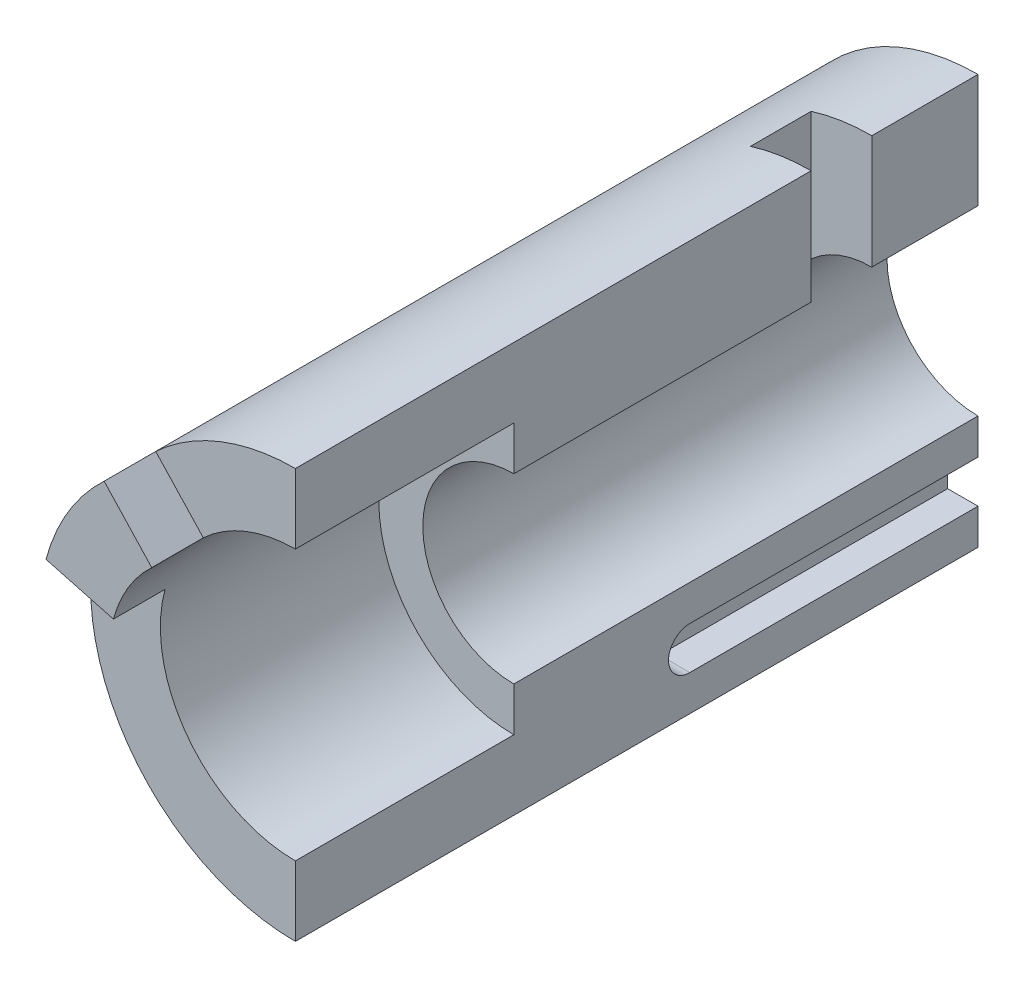
ISO-10303-21;
HEADER;
FILE_DESCRIPTION(('STEP AP214'),'2;1');
FILE_NAME('part.step','',(''),(''),'','','');
FILE_SCHEMA(('AUTOMOTIVE_DESIGN { 1 0 10303 214 1 1 1 1 }'));
ENDSEC;
DATA;
#1=APPLICATION_CONTEXT('core data for automotive mechanical design processes');
#2=APPLICATION_PROTOCOL_DEFINITION('international standard','automotive_design',2000,#1);
#3=PRODUCT_CONTEXT('',#1,'mechanical');
#4=PRODUCT('Part','Part','',(#3));
#5=PRODUCT_RELATED_PRODUCT_CATEGORY('part','',(#4));
#6=PRODUCT_DEFINITION_FORMATION('','',#4);
#7=PRODUCT_DEFINITION_CONTEXT('part definition',#1,'design');
#8=PRODUCT_DEFINITION('design','',#6,#7);
#9=PRODUCT_DEFINITION_SHAPE('','',#8);
#10=(LENGTH_UNIT() NAMED_UNIT(*) SI_UNIT(.MILLI.,.METRE.));
#11=(NAMED_UNIT(*) PLANE_ANGLE_UNIT() SI_UNIT($,.RADIAN.));
#12=(NAMED_UNIT(*) SI_UNIT($,.STERADIAN.) SOLID_ANGLE_UNIT());
#13=UNCERTAINTY_MEASURE_WITH_UNIT(LENGTH_MEASURE(1.E-05),#10,'distance_accuracy_value','');
#14=(GEOMETRIC_REPRESENTATION_CONTEXT(3) GLOBAL_UNCERTAINTY_ASSIGNED_CONTEXT((#13)) GLOBAL_UNIT_ASSIGNED_CONTEXT((#10,
#11,#12)) REPRESENTATION_CONTEXT('',''));
#15=CARTESIAN_POINT('',(0.,0.,0.));
#16=DIRECTION('',(0.,0.,1.));
#17=DIRECTION('',(1.,0.,0.));
#18=AXIS2_PLACEMENT_3D('',#15,#16,#17);
#19=CARTESIAN_POINT('',(0.,0.,-225.));
#20=DIRECTION('',(0.,0.,1.));
#21=DIRECTION('',(1.,0.,0.));
#22=AXIS2_PLACEMENT_3D('',#19,#20,#21);
#23=CYLINDRICAL_SURFACE('',#22,30.);
#24=DIRECTION('',(0.,0.,1.));
#25=VECTOR('',#24,1.);
#26=CARTESIAN_POINT('',(0.,30.,-225.));
#27=LINE('',#26,#25);
#28=CARTESIAN_POINT('',(0.,30.,-225.));
#29=VERTEX_POINT('',#28);
#30=CARTESIAN_POINT('',(0.,30.,-190.));
#31=VERTEX_POINT('',#30);
#32=EDGE_CURVE('E288',#29,#31,#27,.T.);
#33=ORIENTED_EDGE('',*,*,#32,.T.);
#34=CARTESIAN_POINT('',(0.,0.,-190.));
#35=DIRECTION('',(0.,0.,1.));
#36=DIRECTION('',(1.,0.,0.));
#37=AXIS2_PLACEMENT_3D('',#34,#35,#36);
#38=CIRCLE('',#37,30.);
#39=CARTESIAN_POINT('',(-20.,22.3606797749979,-190.));
#40=VERTEX_POINT('',#39);
#41=EDGE_CURVE('E207',#31,#40,#38,.T.);
#42=ORIENTED_EDGE('',*,*,#41,.T.);
#43=DIRECTION('',(0.,0.,1.));
#44=VECTOR('',#43,1.);
#45=CARTESIAN_POINT('',(-20.,22.3606797749979,-225.));
#46=LINE('',#45,#44);
#47=CARTESIAN_POINT('',(-20.,22.3606797749979,-170.));
#48=VERTEX_POINT('',#47);
#49=EDGE_CURVE('E209',#40,#48,#46,.T.);
#50=ORIENTED_EDGE('',*,*,#49,.T.);
#51=CARTESIAN_POINT('',(0.,0.,-170.));
#52=DIRECTION('',(0.,0.,-1.));
#53=DIRECTION('',(-1.,0.,0.));
#54=AXIS2_PLACEMENT_3D('',#51,#52,#53);
#55=CIRCLE('',#54,30.);
#56=CARTESIAN_POINT('',(0.,30.,-170.));
#57=VERTEX_POINT('',#56);
#58=EDGE_CURVE('E199',#48,#57,#55,.T.);
#59=ORIENTED_EDGE('',*,*,#58,.T.);
#60=CARTESIAN_POINT('',(0.,30.,-72.));
#61=VERTEX_POINT('',#60);
#62=EDGE_CURVE('E269',#57,#61,#27,.T.);
#63=ORIENTED_EDGE('',*,*,#62,.T.);
#64=CARTESIAN_POINT('',(0.,0.,-72.));
#65=DIRECTION('',(0.,0.,-1.));
#66=DIRECTION('',(-1.,0.,0.));
#67=AXIS2_PLACEMENT_3D('',#64,#65,#66);
#68=CIRCLE('',#67,30.);
#69=CARTESIAN_POINT('',(0.,-30.,-72.));
#70=VERTEX_POINT('',#69);
#71=EDGE_CURVE('E249',#70,#61,#68,.T.);
#72=ORIENTED_EDGE('',*,*,#71,.F.);
#73=DIRECTION('',(0.,0.,1.));
#74=VECTOR('',#73,1.);
#75=CARTESIAN_POINT('',(0.,-30.,-225.));
#76=LINE('',#75,#74);
#77=CARTESIAN_POINT('',(0.,-30.,-225.));
#78=VERTEX_POINT('',#77);
#79=EDGE_CURVE('E279',#78,#70,#76,.T.);
#80=ORIENTED_EDGE('',*,*,#79,.F.);
#81=CARTESIAN_POINT('',(0.,0.,-225.));
#82=DIRECTION('',(0.,0.,-1.));
#83=DIRECTION('',(1.,0.,0.));
#84=AXIS2_PLACEMENT_3D('',#81,#82,#83);
#85=CIRCLE('',#84,30.);
#86=EDGE_CURVE('E257',#78,#29,#85,.T.);
#87=ORIENTED_EDGE('',*,*,#86,.T.);
#88=EDGE_LOOP('',(#33,#42,#50,#59,#63,#72,#80,#87));
#89=FACE_BOUND('',#88,.T.);
#90=ADVANCED_FACE('F39',(#89),#23,.F.);
#91=CARTESIAN_POINT('',(0.,0.,-225.));
#92=DIRECTION('',(0.,0.,1.));
#93=DIRECTION('',(1.,0.,0.));
#94=AXIS2_PLACEMENT_3D('',#91,#92,#93);
#95=CYLINDRICAL_SURFACE('',#94,67.5);
#96=DIRECTION('',(0.,0.,1.));
#97=VECTOR('',#96,1.);
#98=CARTESIAN_POINT('',(-20.,64.4689847911381,-225.));
#99=LINE('',#98,#97);
#100=CARTESIAN_POINT('',(-20.,64.4689847911381,-170.));
#101=VERTEX_POINT('',#100);
#102=CARTESIAN_POINT('',(-20.,64.4689847911381,-190.));
#103=VERTEX_POINT('',#102);
#104=EDGE_CURVE('E296',#101,#103,#99,.F.);
#105=ORIENTED_EDGE('',*,*,#104,.T.);
#106=CARTESIAN_POINT('',(0.,0.,-190.));
#107=DIRECTION('',(0.,0.,1.));
#108=DIRECTION('',(1.,0.,0.));
#109=AXIS2_PLACEMENT_3D('',#106,#107,#108);
#110=CIRCLE('',#109,67.5);
#111=CARTESIAN_POINT('',(0.,67.5,-190.));
#112=VERTEX_POINT('',#111);
#113=EDGE_CURVE('E202',#103,#112,#110,.F.);
#114=ORIENTED_EDGE('',*,*,#113,.T.);
#115=DIRECTION('',(0.,0.,1.));
#116=VECTOR('',#115,1.);
#117=CARTESIAN_POINT('',(0.,67.5,-225.));
#118=LINE('',#117,#116);
#119=CARTESIAN_POINT('',(0.,67.5,-225.));
#120=VERTEX_POINT('',#119);
#121=EDGE_CURVE('E284',#120,#112,#118,.T.);
#122=ORIENTED_EDGE('',*,*,#121,.F.);
#123=CARTESIAN_POINT('',(0.,0.,-225.));
#124=DIRECTION('',(0.,0.,1.));
#125=DIRECTION('',(1.,0.,0.));
#126=AXIS2_PLACEMENT_3D('',#123,#124,#125);
#127=CIRCLE('',#126,67.5);
#128=CARTESIAN_POINT('',(0.,-67.5,-225.));
#129=VERTEX_POINT('',#128);
#130=EDGE_CURVE('E263',#120,#129,#127,.T.);
#131=ORIENTED_EDGE('',*,*,#130,.T.);
#132=DIRECTION('',(0.,0.,1.));
#133=VECTOR('',#132,1.);
#134=CARTESIAN_POINT('',(0.,-67.5,-225.));
#135=LINE('',#134,#133);
#136=CARTESIAN_POINT('',(0.,-67.5,0.));
#137=VERTEX_POINT('',#136);
#138=EDGE_CURVE('E285',#129,#137,#135,.T.);
#139=ORIENTED_EDGE('',*,*,#138,.T.);
#140=CARTESIAN_POINT('',(0.,0.,0.));
#141=DIRECTION('',(0.,0.,1.));
#142=DIRECTION('',(1.,0.,0.));
#143=AXIS2_PLACEMENT_3D('',#140,#141,#142);
#144=CIRCLE('',#143,67.5);
#145=CARTESIAN_POINT('',(-65.1999932745122,17.47028554442,0.));
#146=VERTEX_POINT('',#145);
#147=EDGE_CURVE('E271',#146,#137,#144,.T.);
#148=ORIENTED_EDGE('',*,*,#147,.F.);
#149=DIRECTION('',(0.,0.,-1.));
#150=VECTOR('',#149,1.);
#151=CARTESIAN_POINT('',(-65.1999932745122,17.47028554442,17.));
#152=LINE('',#151,#150);
#153=CARTESIAN_POINT('',(-65.1999932745122,17.47028554442,17.));
#154=VERTEX_POINT('',#153);
#155=EDGE_CURVE('E236',#154,#146,#152,.T.);
#156=ORIENTED_EDGE('',*,*,#155,.F.);
#157=CARTESIAN_POINT('',(0.,0.,17.));
#158=DIRECTION('',(0.,0.,1.));
#159=DIRECTION('',(1.,0.,0.));
#160=AXIS2_PLACEMENT_3D('',#157,#158,#159);
#161=CIRCLE('',#160,67.5);
#162=CARTESIAN_POINT('',(-46.0348893042187,49.366374859294,17.));
#163=VERTEX_POINT('',#162);
#164=EDGE_CURVE('E214',#163,#154,#161,.T.);
#165=ORIENTED_EDGE('',*,*,#164,.F.);
#166=DIRECTION('',(0.,0.,-1.));
#167=VECTOR('',#166,1.);
#168=CARTESIAN_POINT('',(-46.0348893042187,49.366374859294,17.));
#169=LINE('',#168,#167);
#170=CARTESIAN_POINT('',(-46.0348893042187,49.3663748592939,0.));
#171=VERTEX_POINT('',#170);
#172=EDGE_CURVE('E222',#163,#171,#169,.T.);
#173=ORIENTED_EDGE('',*,*,#172,.T.);
#174=CARTESIAN_POINT('',(0.,67.5,0.));
#175=VERTEX_POINT('',#174);
#176=EDGE_CURVE('E274',#175,#171,#144,.T.);
#177=ORIENTED_EDGE('',*,*,#176,.F.);
#178=CARTESIAN_POINT('',(0.,67.5,-170.));
#179=VERTEX_POINT('',#178);
#180=EDGE_CURVE('E287',#179,#175,#118,.T.);
#181=ORIENTED_EDGE('',*,*,#180,.F.);
#182=CARTESIAN_POINT('',(0.,0.,-170.));
#183=DIRECTION('',(0.,0.,-1.));
#184=DIRECTION('',(-1.,0.,0.));
#185=AXIS2_PLACEMENT_3D('',#182,#183,#184);
#186=CIRCLE('',#185,67.5);
#187=EDGE_CURVE('E62',#179,#101,#186,.F.);
#188=ORIENTED_EDGE('',*,*,#187,.T.);
#189=EDGE_LOOP('',(#105,#114,#122,#131,#139,#148,#156,#165,#173,#177,#181,#188));
#190=FACE_BOUND('',#189,.T.);
#191=ADVANCED_FACE('F336',(#190),#95,.T.);
#192=CARTESIAN_POINT('',(0.,67.5,-225.));
#193=DIRECTION('',(1.,0.,0.));
#194=DIRECTION('',(0.,0.,-1.));
#195=AXIS2_PLACEMENT_3D('',#192,#193,#194);
#196=PLANE('',#195);
#197=ORIENTED_EDGE('',*,*,#121,.T.);
#198=DIRECTION('',(0.,-1.,0.));
#199=VECTOR('',#198,1.);
#200=CARTESIAN_POINT('',(0.,67.5,-190.));
#201=LINE('',#200,#199);
#202=EDGE_CURVE('E294',#112,#31,#201,.T.);
#203=ORIENTED_EDGE('',*,*,#202,.T.);
#204=ORIENTED_EDGE('',*,*,#32,.F.);
#205=DIRECTION('',(0.,1.,0.));
#206=VECTOR('',#205,1.);
#207=CARTESIAN_POINT('',(0.,67.5,-225.));
#208=LINE('',#207,#206);
#209=EDGE_CURVE('E256',#29,#120,#208,.T.);
#210=ORIENTED_EDGE('',*,*,#209,.T.);
#211=EDGE_LOOP('',(#197,#203,#204,#210));
#212=FACE_BOUND('',#211,.T.);
#213=ADVANCED_FACE('F317',(#212),#196,.T.);
#214=ORIENTED_EDGE('',*,*,#62,.F.);
#215=DIRECTION('',(0.,1.,0.));
#216=VECTOR('',#215,1.);
#217=CARTESIAN_POINT('',(0.,67.5,-170.));
#218=LINE('',#217,#216);
#219=EDGE_CURVE('E291',#57,#179,#218,.T.);
#220=ORIENTED_EDGE('',*,*,#219,.T.);
#221=ORIENTED_EDGE('',*,*,#180,.T.);
#222=DIRECTION('',(0.,1.,0.));
#223=VECTOR('',#222,1.);
#224=CARTESIAN_POINT('',(0.,67.5,0.));
#225=LINE('',#224,#223);
#226=CARTESIAN_POINT('',(0.,44.5,0.));
#227=VERTEX_POINT('',#226);
#228=EDGE_CURVE('E253',#227,#175,#225,.T.);
#229=ORIENTED_EDGE('',*,*,#228,.F.);
#230=DIRECTION('',(0.,0.,1.));
#231=VECTOR('',#230,1.);
#232=CARTESIAN_POINT('',(0.,44.5,32.7369619908887));
#233=LINE('',#232,#231);
#234=CARTESIAN_POINT('',(0.,44.5,-72.));
#235=VERTEX_POINT('',#234);
#236=EDGE_CURVE('E246',#235,#227,#233,.T.);
#237=ORIENTED_EDGE('',*,*,#236,.F.);
#238=DIRECTION('',(0.,1.,0.));
#239=VECTOR('',#238,1.);
#240=CARTESIAN_POINT('',(0.,67.5,-72.));
#241=LINE('',#240,#239);
#242=EDGE_CURVE('E281',#61,#235,#241,.T.);
#243=ORIENTED_EDGE('',*,*,#242,.F.);
#244=EDGE_LOOP('',(#214,#220,#221,#229,#237,#243));
#245=FACE_BOUND('',#244,.T.);
#246=ADVANCED_FACE('F332',(#245),#196,.T.);
#247=CARTESIAN_POINT('',(0.,0.,0.));
#248=DIRECTION('',(0.,0.,1.));
#249=DIRECTION('',(1.,0.,0.));
#250=AXIS2_PLACEMENT_3D('',#247,#248,#249);
#251=PLANE('',#250);
#252=DIRECTION('',(-0.6819983600625,0.731353701619169,0.));
#253=VECTOR('',#252,1.);
#254=CARTESIAN_POINT('',(-30.3489270227812,32.545239722053,0.));
#255=LINE('',#254,#253);
#256=CARTESIAN_POINT('',(-30.3489270227812,32.545239722053,0.));
#257=VERTEX_POINT('',#256);
#258=EDGE_CURVE('E220',#257,#171,#255,.T.);
#259=ORIENTED_EDGE('',*,*,#258,.F.);
#260=CARTESIAN_POINT('',(0.,0.,0.));
#261=DIRECTION('',(0.,0.,1.));
#262=DIRECTION('',(1.,0.,0.));
#263=AXIS2_PLACEMENT_3D('',#260,#261,#262);
#264=CIRCLE('',#263,44.5);
#265=EDGE_CURVE('E239',#227,#257,#264,.T.);
#266=ORIENTED_EDGE('',*,*,#265,.F.);
#267=ORIENTED_EDGE('',*,*,#228,.T.);
#268=ORIENTED_EDGE('',*,*,#176,.T.);
#269=EDGE_LOOP('',(#259,#266,#267,#268));
#270=FACE_BOUND('',#269,.T.);
#271=ADVANCED_FACE('F340',(#270),#251,.T.);
#272=CARTESIAN_POINT('',(0.,-30.,-225.));
#273=DIRECTION('',(1.,0.,0.));
#274=DIRECTION('',(0.,0.,-1.));
#275=AXIS2_PLACEMENT_3D('',#272,#273,#274);
#276=PLANE('',#275);
#277=DIRECTION('',(0.,0.,-1.));
#278=VECTOR('',#277,1.);
#279=CARTESIAN_POINT('',(0.,-55.75,-239.283215377348));
#280=LINE('',#279,#278);
#281=CARTESIAN_POINT('',(0.,-55.75,-130.));
#282=VERTEX_POINT('',#281);
#283=CARTESIAN_POINT('',(0.,-55.75,-225.));
#284=VERTEX_POINT('',#283);
#285=EDGE_CURVE('E175',#282,#284,#280,.T.);
#286=ORIENTED_EDGE('',*,*,#285,.F.);
#287=CARTESIAN_POINT('',(0.,-48.75,-130.));
#288=DIRECTION('',(1.,0.,0.));
#289=DIRECTION('',(0.,0.,-1.));
#290=AXIS2_PLACEMENT_3D('',#287,#288,#289);
#291=CIRCLE('',#290,7.);
#292=CARTESIAN_POINT('',(0.,-41.75,-130.));
#293=VERTEX_POINT('',#292);
#294=EDGE_CURVE('E186',#293,#282,#291,.T.);
#295=ORIENTED_EDGE('',*,*,#294,.F.);
#296=DIRECTION('',(0.,0.,1.));
#297=VECTOR('',#296,1.);
#298=CARTESIAN_POINT('',(0.,-41.75,-239.283215377348));
#299=LINE('',#298,#297);
#300=CARTESIAN_POINT('',(0.,-41.75,-225.));
#301=VERTEX_POINT('',#300);
#302=EDGE_CURVE('E178',#301,#293,#299,.T.);
#303=ORIENTED_EDGE('',*,*,#302,.F.);
#304=DIRECTION('',(0.,1.,0.));
#305=VECTOR('',#304,1.);
#306=CARTESIAN_POINT('',(0.,-30.,-225.));
#307=LINE('',#306,#305);
#308=EDGE_CURVE('E266',#301,#78,#307,.T.);
#309=ORIENTED_EDGE('',*,*,#308,.T.);
#310=ORIENTED_EDGE('',*,*,#79,.T.);
#311=DIRECTION('',(0.,1.,0.));
#312=VECTOR('',#311,1.);
#313=CARTESIAN_POINT('',(0.,-30.,-72.));
#314=LINE('',#313,#312);
#315=CARTESIAN_POINT('',(0.,-44.5,-72.));
#316=VERTEX_POINT('',#315);
#317=EDGE_CURVE('E254',#316,#70,#314,.T.);
#318=ORIENTED_EDGE('',*,*,#317,.F.);
#319=DIRECTION('',(0.,0.,1.));
#320=VECTOR('',#319,1.);
#321=CARTESIAN_POINT('',(0.,-44.5,32.7369619908887));
#322=LINE('',#321,#320);
#323=CARTESIAN_POINT('',(0.,-44.5,0.));
#324=VERTEX_POINT('',#323);
#325=EDGE_CURVE('E247',#324,#316,#322,.F.);
#326=ORIENTED_EDGE('',*,*,#325,.F.);
#327=DIRECTION('',(0.,1.,0.));
#328=VECTOR('',#327,1.);
#329=CARTESIAN_POINT('',(0.,-30.,0.));
#330=LINE('',#329,#328);
#331=EDGE_CURVE('E258',#137,#324,#330,.T.);
#332=ORIENTED_EDGE('',*,*,#331,.F.);
#333=ORIENTED_EDGE('',*,*,#138,.F.);
#334=EDGE_CURVE('E270',#129,#284,#307,.T.);
#335=ORIENTED_EDGE('',*,*,#334,.T.);
#336=EDGE_LOOP('',(#286,#295,#303,#309,#310,#318,#326,#332,#333,#335));
#337=FACE_BOUND('',#336,.T.);
#338=ADVANCED_FACE('F310',(#337),#276,.T.);
#339=CARTESIAN_POINT('',(0.,0.,-225.));
#340=DIRECTION('',(0.,0.,1.));
#341=DIRECTION('',(1.,0.,0.));
#342=AXIS2_PLACEMENT_3D('',#339,#340,#341);
#343=PLANE('',#342);
#344=DIRECTION('',(0.,1.,0.));
#345=VECTOR('',#344,1.);
#346=CARTESIAN_POINT('',(-10.,0.,-225.));
#347=LINE('',#346,#345);
#348=CARTESIAN_POINT('',(-10.,-55.75,-225.));
#349=VERTEX_POINT('',#348);
#350=CARTESIAN_POINT('',(-10.,-41.75,-225.));
#351=VERTEX_POINT('',#350);
#352=EDGE_CURVE('E169',#349,#351,#347,.T.);
#353=ORIENTED_EDGE('',*,*,#352,.F.);
#354=DIRECTION('',(1.,0.,0.));
#355=VECTOR('',#354,1.);
#356=CARTESIAN_POINT('',(0.,-55.75,-225.));
#357=LINE('',#356,#355);
#358=EDGE_CURVE('E11',#349,#284,#357,.T.);
#359=ORIENTED_EDGE('',*,*,#358,.T.);
#360=ORIENTED_EDGE('',*,*,#334,.F.);
#361=ORIENTED_EDGE('',*,*,#130,.F.);
#362=ORIENTED_EDGE('',*,*,#209,.F.);
#363=ORIENTED_EDGE('',*,*,#86,.F.);
#364=ORIENTED_EDGE('',*,*,#308,.F.);
#365=DIRECTION('',(-1.,0.,0.));
#366=VECTOR('',#365,1.);
#367=CARTESIAN_POINT('',(0.,-41.75,-225.));
#368=LINE('',#367,#366);
#369=EDGE_CURVE('E46',#301,#351,#368,.T.);
#370=ORIENTED_EDGE('',*,*,#369,.T.);
#371=EDGE_LOOP('',(#353,#359,#360,#361,#362,#363,#364,#370));
#372=FACE_BOUND('',#371,.T.);
#373=ADVANCED_FACE('F303',(#372),#343,.F.);
#374=DIRECTION('',(0.965925826289069,-0.258819045102519,0.));
#375=VECTOR('',#374,1.);
#376=CARTESIAN_POINT('',(-42.9836992698636,11.5174475070621,0.));
#377=LINE('',#376,#375);
#378=CARTESIAN_POINT('',(-42.9836992698636,11.5174475070621,0.));
#379=VERTEX_POINT('',#378);
#380=EDGE_CURVE('E215',#146,#379,#377,.T.);
#381=ORIENTED_EDGE('',*,*,#380,.F.);
#382=ORIENTED_EDGE('',*,*,#147,.T.);
#383=ORIENTED_EDGE('',*,*,#331,.T.);
#384=EDGE_CURVE('E237',#379,#324,#264,.T.);
#385=ORIENTED_EDGE('',*,*,#384,.F.);
#386=EDGE_LOOP('',(#381,#382,#383,#385));
#387=FACE_BOUND('',#386,.T.);
#388=ADVANCED_FACE('F353',(#387),#251,.T.);
#389=CARTESIAN_POINT('',(0.,0.,-72.));
#390=DIRECTION('',(0.,0.,-1.));
#391=DIRECTION('',(-1.,0.,0.));
#392=AXIS2_PLACEMENT_3D('',#389,#390,#391);
#393=PLANE('',#392);
#394=ORIENTED_EDGE('',*,*,#317,.T.);
#395=ORIENTED_EDGE('',*,*,#71,.T.);
#396=ORIENTED_EDGE('',*,*,#242,.T.);
#397=CARTESIAN_POINT('',(0.,0.,-72.));
#398=DIRECTION('',(0.,0.,1.));
#399=DIRECTION('',(1.,0.,0.));
#400=AXIS2_PLACEMENT_3D('',#397,#398,#399);
#401=CIRCLE('',#400,44.5);
#402=EDGE_CURVE('E243',#235,#316,#401,.T.);
#403=ORIENTED_EDGE('',*,*,#402,.T.);
#404=EDGE_LOOP('',(#394,#395,#396,#403));
#405=FACE_BOUND('',#404,.T.);
#406=ADVANCED_FACE('F324',(#405),#393,.F.);
#407=CARTESIAN_POINT('',(0.,0.,32.7369619908887));
#408=DIRECTION('',(0.,0.,1.));
#409=DIRECTION('',(1.,0.,0.));
#410=AXIS2_PLACEMENT_3D('',#407,#408,#409);
#411=CYLINDRICAL_SURFACE('',#410,44.5);
#412=ORIENTED_EDGE('',*,*,#325,.T.);
#413=ORIENTED_EDGE('',*,*,#402,.F.);
#414=ORIENTED_EDGE('',*,*,#236,.T.);
#415=ORIENTED_EDGE('',*,*,#265,.T.);
#416=DIRECTION('',(0.,0.,-1.));
#417=VECTOR('',#416,1.);
#418=CARTESIAN_POINT('',(-30.3489270227812,32.545239722053,17.));
#419=LINE('',#418,#417);
#420=CARTESIAN_POINT('',(-30.3489270227812,32.545239722053,17.));
#421=VERTEX_POINT('',#420);
#422=EDGE_CURVE('E229',#421,#257,#419,.T.);
#423=ORIENTED_EDGE('',*,*,#422,.F.);
#424=CARTESIAN_POINT('',(0.,0.,17.));
#425=DIRECTION('',(0.,0.,-1.));
#426=DIRECTION('',(1.,0.,0.));
#427=AXIS2_PLACEMENT_3D('',#424,#425,#426);
#428=CIRCLE('',#427,44.5);
#429=CARTESIAN_POINT('',(-42.9836992698636,11.5174475070621,17.));
#430=VERTEX_POINT('',#429);
#431=EDGE_CURVE('E217',#430,#421,#428,.T.);
#432=ORIENTED_EDGE('',*,*,#431,.F.);
#433=DIRECTION('',(0.,0.,-1.));
#434=VECTOR('',#433,1.);
#435=CARTESIAN_POINT('',(-42.9836992698636,11.5174475070621,17.));
#436=LINE('',#435,#434);
#437=EDGE_CURVE('E231',#430,#379,#436,.T.);
#438=ORIENTED_EDGE('',*,*,#437,.T.);
#439=ORIENTED_EDGE('',*,*,#384,.T.);
#440=EDGE_LOOP('',(#412,#413,#414,#415,#423,#432,#438,#439));
#441=FACE_BOUND('',#440,.T.);
#442=ADVANCED_FACE('F328',(#441),#411,.F.);
#443=CARTESIAN_POINT('',(-42.9836992698636,11.5174475070621,17.));
#444=DIRECTION('',(0.258819045102519,0.965925826289069,0.));
#445=DIRECTION('',(-0.965925826289069,0.258819045102519,0.));
#446=AXIS2_PLACEMENT_3D('',#443,#444,#445);
#447=PLANE('',#446);
#448=ORIENTED_EDGE('',*,*,#380,.T.);
#449=ORIENTED_EDGE('',*,*,#437,.F.);
#450=DIRECTION('',(0.965925826289069,-0.258819045102519,0.));
#451=VECTOR('',#450,1.);
#452=CARTESIAN_POINT('',(-42.9836992698636,11.5174475070621,17.));
#453=LINE('',#452,#451);
#454=EDGE_CURVE('E216',#154,#430,#453,.T.);
#455=ORIENTED_EDGE('',*,*,#454,.F.);
#456=ORIENTED_EDGE('',*,*,#155,.T.);
#457=EDGE_LOOP('',(#448,#449,#455,#456));
#458=FACE_BOUND('',#457,.T.);
#459=ADVANCED_FACE('F351',(#458),#447,.F.);
#460=CARTESIAN_POINT('',(-30.3489270227812,32.545239722053,17.));
#461=DIRECTION('',(-0.731353701619169,-0.6819983600625,0.));
#462=DIRECTION('',(0.6819983600625,-0.731353701619169,0.));
#463=AXIS2_PLACEMENT_3D('',#460,#461,#462);
#464=PLANE('',#463);
#465=ORIENTED_EDGE('',*,*,#258,.T.);
#466=ORIENTED_EDGE('',*,*,#172,.F.);
#467=DIRECTION('',(-0.6819983600625,0.731353701619169,0.));
#468=VECTOR('',#467,1.);
#469=CARTESIAN_POINT('',(-30.3489270227812,32.545239722053,17.));
#470=LINE('',#469,#468);
#471=EDGE_CURVE('E221',#421,#163,#470,.T.);
#472=ORIENTED_EDGE('',*,*,#471,.F.);
#473=ORIENTED_EDGE('',*,*,#422,.T.);
#474=EDGE_LOOP('',(#465,#466,#472,#473));
#475=FACE_BOUND('',#474,.T.);
#476=ADVANCED_FACE('F341',(#475),#464,.F.);
#477=CARTESIAN_POINT('',(0.,0.,17.));
#478=DIRECTION('',(0.,0.,1.));
#479=DIRECTION('',(1.,0.,0.));
#480=AXIS2_PLACEMENT_3D('',#477,#478,#479);
#481=PLANE('',#480);
#482=ORIENTED_EDGE('',*,*,#164,.T.);
#483=ORIENTED_EDGE('',*,*,#454,.T.);
#484=ORIENTED_EDGE('',*,*,#431,.T.);
#485=ORIENTED_EDGE('',*,*,#471,.T.);
#486=EDGE_LOOP('',(#482,#483,#484,#485));
#487=FACE_BOUND('',#486,.T.);
#488=ADVANCED_FACE('F347',(#487),#481,.T.);
#489=CARTESIAN_POINT('',(0.,97.,-190.));
#490=DIRECTION('',(0.,0.,1.));
#491=DIRECTION('',(1.,0.,0.));
#492=AXIS2_PLACEMENT_3D('',#489,#490,#491);
#493=PLANE('',#492);
#494=ORIENTED_EDGE('',*,*,#202,.F.);
#495=ORIENTED_EDGE('',*,*,#113,.F.);
#496=DIRECTION('',(0.,-1.,0.));
#497=VECTOR('',#496,1.);
#498=CARTESIAN_POINT('',(-20.,97.,-190.));
#499=LINE('',#498,#497);
#500=EDGE_CURVE('E196',#103,#40,#499,.T.);
#501=ORIENTED_EDGE('',*,*,#500,.T.);
#502=ORIENTED_EDGE('',*,*,#41,.F.);
#503=EDGE_LOOP('',(#494,#495,#501,#502));
#504=FACE_BOUND('',#503,.T.);
#505=ADVANCED_FACE('F433',(#504),#493,.T.);
#506=CARTESIAN_POINT('',(-20.,97.,-190.));
#507=DIRECTION('',(1.,0.,0.));
#508=DIRECTION('',(0.,0.,-1.));
#509=AXIS2_PLACEMENT_3D('',#506,#507,#508);
#510=PLANE('',#509);
#511=ORIENTED_EDGE('',*,*,#500,.F.);
#512=ORIENTED_EDGE('',*,*,#104,.F.);
#513=DIRECTION('',(0.,-1.,0.));
#514=VECTOR('',#513,1.);
#515=CARTESIAN_POINT('',(-20.,97.,-170.));
#516=LINE('',#515,#514);
#517=EDGE_CURVE('E195',#101,#48,#516,.T.);
#518=ORIENTED_EDGE('',*,*,#517,.T.);
#519=ORIENTED_EDGE('',*,*,#49,.F.);
#520=EDGE_LOOP('',(#511,#512,#518,#519));
#521=FACE_BOUND('',#520,.T.);
#522=ADVANCED_FACE('F428',(#521),#510,.T.);
#523=CARTESIAN_POINT('',(0.,97.,-170.));
#524=DIRECTION('',(0.,0.,-1.));
#525=DIRECTION('',(-1.,0.,0.));
#526=AXIS2_PLACEMENT_3D('',#523,#524,#525);
#527=PLANE('',#526);
#528=ORIENTED_EDGE('',*,*,#517,.F.);
#529=ORIENTED_EDGE('',*,*,#187,.F.);
#530=ORIENTED_EDGE('',*,*,#219,.F.);
#531=ORIENTED_EDGE('',*,*,#58,.F.);
#532=EDGE_LOOP('',(#528,#529,#530,#531));
#533=FACE_BOUND('',#532,.T.);
#534=ADVANCED_FACE('F384',(#533),#527,.T.);
#535=CARTESIAN_POINT('',(-10.,-55.75,-239.283215377348));
#536=DIRECTION('',(0.,-1.,0.));
#537=DIRECTION('',(0.,0.,-1.));
#538=AXIS2_PLACEMENT_3D('',#535,#536,#537);
#539=PLANE('',#538);
#540=DIRECTION('',(0.,0.,-1.));
#541=VECTOR('',#540,1.);
#542=CARTESIAN_POINT('',(-10.,-55.75,-239.283215377348));
#543=LINE('',#542,#541);
#544=CARTESIAN_POINT('',(-10.,-55.75,-130.));
#545=VERTEX_POINT('',#544);
#546=EDGE_CURVE('E52',#545,#349,#543,.T.);
#547=ORIENTED_EDGE('',*,*,#546,.F.);
#548=DIRECTION('',(1.,0.,0.));
#549=VECTOR('',#548,1.);
#550=CARTESIAN_POINT('',(-10.,-55.75,-130.));
#551=LINE('',#550,#549);
#552=EDGE_CURVE('E185',#545,#282,#551,.T.);
#553=ORIENTED_EDGE('',*,*,#552,.T.);
#554=ORIENTED_EDGE('',*,*,#285,.T.);
#555=ORIENTED_EDGE('',*,*,#358,.F.);
#556=EDGE_LOOP('',(#547,#553,#554,#555));
#557=FACE_BOUND('',#556,.T.);
#558=ADVANCED_FACE('F311',(#557),#539,.F.);
#559=CARTESIAN_POINT('',(-10.,-41.75,-239.283215377348));
#560=DIRECTION('',(0.,1.,0.));
#561=DIRECTION('',(0.,0.,1.));
#562=AXIS2_PLACEMENT_3D('',#559,#560,#561);
#563=PLANE('',#562);
#564=ORIENTED_EDGE('',*,*,#302,.T.);
#565=DIRECTION('',(1.,0.,0.));
#566=VECTOR('',#565,1.);
#567=CARTESIAN_POINT('',(-10.,-41.75,-130.));
#568=LINE('',#567,#566);
#569=CARTESIAN_POINT('',(-10.,-41.75,-130.));
#570=VERTEX_POINT('',#569);
#571=EDGE_CURVE('E174',#570,#293,#568,.T.);
#572=ORIENTED_EDGE('',*,*,#571,.F.);
#573=DIRECTION('',(0.,0.,1.));
#574=VECTOR('',#573,1.);
#575=CARTESIAN_POINT('',(-10.,-41.75,-239.283215377348));
#576=LINE('',#575,#574);
#577=EDGE_CURVE('E161',#351,#570,#576,.T.);
#578=ORIENTED_EDGE('',*,*,#577,.F.);
#579=ORIENTED_EDGE('',*,*,#369,.F.);
#580=EDGE_LOOP('',(#564,#572,#578,#579));
#581=FACE_BOUND('',#580,.T.);
#582=ADVANCED_FACE('F176',(#581),#563,.F.);
#583=CARTESIAN_POINT('',(-10.,-48.75,-239.283215377348));
#584=DIRECTION('',(1.,0.,0.));
#585=DIRECTION('',(0.,0.,-1.));
#586=AXIS2_PLACEMENT_3D('',#583,#584,#585);
#587=PLANE('',#586);
#588=ORIENTED_EDGE('',*,*,#352,.T.);
#589=ORIENTED_EDGE('',*,*,#577,.T.);
#590=CARTESIAN_POINT('',(-10.,-48.75,-130.));
#591=DIRECTION('',(1.,0.,0.));
#592=DIRECTION('',(0.,0.,-1.));
#593=AXIS2_PLACEMENT_3D('',#590,#591,#592);
#594=CIRCLE('',#593,7.);
#595=EDGE_CURVE('E170',#570,#545,#594,.T.);
#596=ORIENTED_EDGE('',*,*,#595,.T.);
#597=ORIENTED_EDGE('',*,*,#546,.T.);
#598=EDGE_LOOP('',(#588,#589,#596,#597));
#599=FACE_BOUND('',#598,.T.);
#600=ADVANCED_FACE('F164',(#599),#587,.T.);
#601=CARTESIAN_POINT('',(-10.,-48.75,-130.));
#602=DIRECTION('',(1.,0.,0.));
#603=DIRECTION('',(0.,0.,-1.));
#604=AXIS2_PLACEMENT_3D('',#601,#602,#603);
#605=CYLINDRICAL_SURFACE('',#604,7.);
#606=ORIENTED_EDGE('',*,*,#294,.T.);
#607=ORIENTED_EDGE('',*,*,#552,.F.);
#608=ORIENTED_EDGE('',*,*,#595,.F.);
#609=ORIENTED_EDGE('',*,*,#571,.T.);
#610=EDGE_LOOP('',(#606,#607,#608,#609));
#611=FACE_BOUND('',#610,.T.);
#612=ADVANCED_FACE('F183',(#611),#605,.F.);
#613=CLOSED_SHELL('',(#90,#191,#213,#246,#271,#338,#373,#388,#406,#442,#459,#476,#488,#505,#522,
#534,#558,#582,#600,#612));
#614=MANIFOLD_SOLID_BREP('B2',#613);
#615=ADVANCED_BREP_SHAPE_REPRESENTATION('',(#18,#614),#14);
#616=SHAPE_DEFINITION_REPRESENTATION(#9,#615);
ENDSEC;
END-ISO-10303-21;
